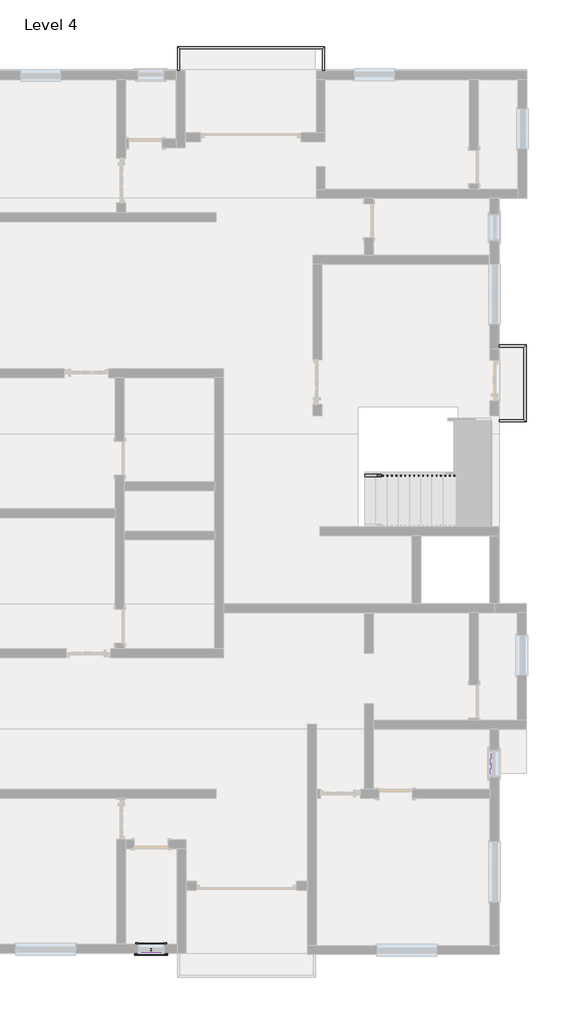
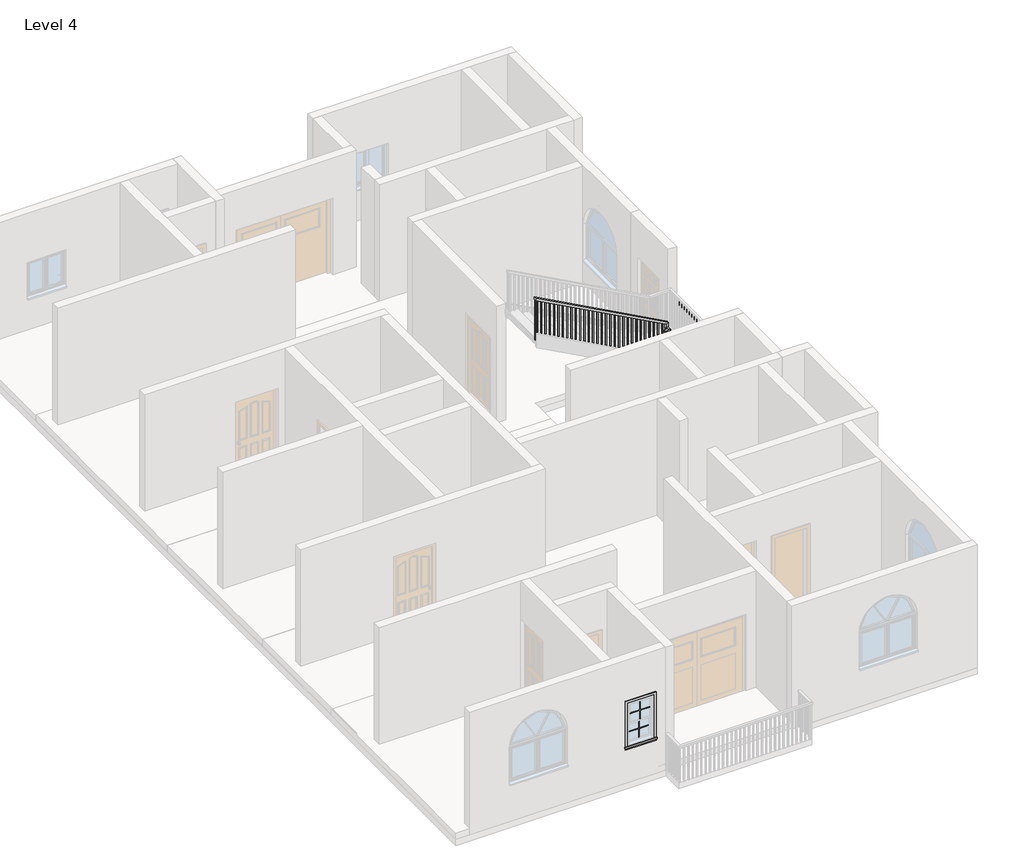
# One storey, part 6 of 7: 5 proxies, 3 railings.
"""IFC4 building model written with IfcOpenShell, lengths in millimetres."""

from ifc_helpers import new_model, si_unit, frame, origin, place, context, project, spatial, polyline, outline, extrude, faceted_brep, transform, mapped, element, save
from components import muntin_pattern_2x2_muntin_pattern_2x2_eba6c5fb, trim_window_exterior_flat_with_sill_278e6a94, trim_window_interior_flat_picture_frame_e9fd5f45

model = new_model("IFC4")

# Units and contexts
model_context = context("Model", 3, world=origin())
ifc_project = project(units=[si_unit("LENGTHUNIT", "METRE", prefix="MILLI")], contexts=[model_context])

# Site, building, storey
site = spatial("IfcSite", under=ifc_project)
building = spatial("IfcBuilding", under=site)
storey = spatial("IfcBuildingStorey", under=building, Name="Level 4", Elevation=9144.0)

# Proxies
placement = place(None, origin())
muntin_pattern_2x2_muntin_pattern_2x2_shape = muntin_pattern_2x2_muntin_pattern_2x2_eba6c5fb(model_context)
element("IfcBuildingElementProxy", 1, Name="Muntin Pattern_2x2 : Muntin Pattern_2x2", ObjectType="Muntin Pattern_2x2 : Muntin Pattern_2x2", at=placement, inside=storey, context=model_context, shape_type="MappedRepresentation", body=[
    mapped(muntin_pattern_2x2_muntin_pattern_2x2_shape, transform((5694.9140963, -6313.9537749, 10614.025), x_axis=(0.0, 1.0, 0.0), y_axis=(-1.0, 0.0, 0.0), z_axis=(0.0, 0.0, 1.0))),
])
element("IfcBuildingElementProxy", 2, Name="Muntin Pattern_2x2 : Muntin Pattern_2x2", ObjectType="Muntin Pattern_2x2 : Muntin Pattern_2x2", at=placement, inside=storey, context=model_context, shape_type="MappedRepresentation", body=[
    mapped(muntin_pattern_2x2_muntin_pattern_2x2_shape, transform((-2023.5109037, -10577.9787749, 10614.025), x_axis=(-1.0, 0.0, 0.0), y_axis=(0.0, -1.0, 0.0), z_axis=(0.0, 0.0, 1.0))),
])
element("IfcBuildingElementProxy", 3, Name="Muntin Pattern_2x2 : Muntin Pattern_2x2", ObjectType="Muntin Pattern_2x2 : Muntin Pattern_2x2", at=placement, inside=storey, context=model_context, shape_type="MappedRepresentation", body=[
    mapped(muntin_pattern_2x2_muntin_pattern_2x2_shape, transform((-2023.5109037, -10533.5287749, 10134.6), x_axis=(-1.0, 0.0, 0.0), y_axis=(0.0, -1.0, 0.0), z_axis=(0.0, 0.0, 1.0))),
])
trim_window_exterior_flat_with_sill_shape = trim_window_exterior_flat_with_sill_278e6a94(model_context)
element("IfcBuildingElementProxy", 4, Name="Trim-Window-Exterior-Flat : with Sill", ObjectType="Trim-Window-Exterior-Flat : with Sill", at=placement, inside=storey, context=model_context, shape_type="MappedRepresentation", body=[
    mapped(trim_window_exterior_flat_with_sill_shape, transform((-2023.5109037, -10612.9037749, 11125.2), x_axis=(1.0, 0.0, 0.0), y_axis=(0.0, 0.0, 1.0), z_axis=(0.0, -1.0, 0.0))),
])
trim_window_interior_flat_picture_frame_shape = trim_window_interior_flat_picture_frame_e9fd5f45(model_context)
element("IfcBuildingElementProxy", 5, Name="Trim-Window-Interior-Flat : Picture Frame", ObjectType="Trim-Window-Interior-Flat : Picture Frame", at=placement, inside=storey, context=model_context, shape_type="MappedRepresentation", body=[
    mapped(trim_window_interior_flat_picture_frame_shape, transform((-2023.5109037, -10409.7037749, 11125.2), x_axis=(-1.0, 0.0, 0.0), y_axis=(0.0, 0.0, 1.0), z_axis=(0.0, 1.0, 0.0))),
])

# Railings
element("IfcRailing", 6, ObjectType="Handrail - Rectangular", at=placement, inside=storey, context=model_context, shape_type="SolidModel", body=[
    faceted_brep([(-1426.6109037, 9402.2962251, 10058.4), (-1426.6109037, 9402.2962251, 10007.6), (-1375.8109037, 9402.2962251, 10007.6), (-1375.8109037, 9402.2962251, 10058.4), (-1426.6109037, 9948.3962251, 10058.4), (-1426.6109037, 9948.3962251, 10007.6), (-1375.8109037, 9897.5962251, 10007.6), (-1375.8109037, 9897.5962251, 10058.4), (1913.4890963, 9948.3962251, 10058.4), (1913.4890963, 9948.3962251, 10007.6), (1862.6890963, 9897.5962251, 10007.6), (1862.6890963, 9897.5962251, 10058.4), (1913.4890963, 9402.2962251, 10058.4), (1862.6890963, 9402.2962251, 10058.4), (1862.6890963, 9402.2962251, 10007.6), (1913.4890963, 9402.2962251, 10007.6)], [[[0, 1, 2, 3]], [[1, 0, 4, 5]], [[2, 1, 5, 6]], [[3, 2, 6, 7]], [[0, 3, 7, 4]], [[5, 4, 8, 9]], [[6, 5, 9, 10]], [[7, 6, 10, 11]], [[4, 7, 11, 8]], [[12, 13, 14, 15]], [[9, 8, 12, 15]], [[10, 9, 15, 14]], [[11, 10, 14, 13]], [[8, 11, 13, 12]]]),
    extrude(outline(polyline([(1878.5640963, 9424.5212251), (1897.6140963, 9424.5212251), (1897.6140963, 9405.4712251), (1878.5640963, 9405.4712251), (1878.5640963, 9424.5212251)])), frame((0.0, 0.0, 9144.0), z_axis=(0.0, 0.0, 1.0), x_axis=(1.0, 0.0, 0.0)), (0.0, 0.0, 1.0), 863.6),
    extrude(outline(polyline([(1878.5640963, 9526.1212251), (1897.6140963, 9526.1212251), (1897.6140963, 9507.0712251), (1878.5640963, 9507.0712251), (1878.5640963, 9526.1212251)])), frame((0.0, 0.0, 9144.0), z_axis=(0.0, 0.0, 1.0), x_axis=(1.0, 0.0, 0.0)), (0.0, 0.0, 1.0), 863.6),
    extrude(outline(polyline([(1878.5640963, 9627.7212251), (1897.6140963, 9627.7212251), (1897.6140963, 9608.6712251), (1878.5640963, 9608.6712251), (1878.5640963, 9627.7212251)])), frame((0.0, 0.0, 9144.0), z_axis=(0.0, 0.0, 1.0), x_axis=(1.0, 0.0, 0.0)), (0.0, 0.0, 1.0), 863.6),
    extrude(outline(polyline([(1878.5640963, 9729.3212251), (1897.6140963, 9729.3212251), (1897.6140963, 9710.2712251), (1878.5640963, 9710.2712251), (1878.5640963, 9729.3212251)])), frame((0.0, 0.0, 9144.0), z_axis=(0.0, 0.0, 1.0), x_axis=(1.0, 0.0, 0.0)), (0.0, 0.0, 1.0), 863.6),
    extrude(outline(polyline([(1878.5640963, 9830.9212251), (1897.6140963, 9830.9212251), (1897.6140963, 9811.8712251), (1878.5640963, 9811.8712251), (1878.5640963, 9830.9212251)])), frame((0.0, 0.0, 9144.0), z_axis=(0.0, 0.0, 1.0), x_axis=(1.0, 0.0, 0.0)), (0.0, 0.0, 1.0), 863.6),
    extrude(outline(polyline([(1840.4640963, 9913.4712251), (1840.4640963, 9932.5212251), (1859.5140963, 9932.5212251), (1859.5140963, 9913.4712251), (1840.4640963, 9913.4712251)])), frame((0.0, 0.0, 9144.0), z_axis=(0.0, 0.0, 1.0), x_axis=(1.0, 0.0, 0.0)), (0.0, 0.0, 1.0), 863.6),
    extrude(outline(polyline([(1738.8640963, 9913.4712251), (1738.8640963, 9932.5212251), (1757.9140963, 9932.5212251), (1757.9140963, 9913.4712251), (1738.8640963, 9913.4712251)])), frame((0.0, 0.0, 9144.0), z_axis=(0.0, 0.0, 1.0), x_axis=(1.0, 0.0, 0.0)), (0.0, 0.0, 1.0), 863.6),
    extrude(outline(polyline([(1637.2640963, 9913.4712251), (1637.2640963, 9932.5212251), (1656.3140963, 9932.5212251), (1656.3140963, 9913.4712251), (1637.2640963, 9913.4712251)])), frame((0.0, 0.0, 9144.0), z_axis=(0.0, 0.0, 1.0), x_axis=(1.0, 0.0, 0.0)), (0.0, 0.0, 1.0), 863.6),
    extrude(outline(polyline([(1535.6640963, 9913.4712251), (1535.6640963, 9932.5212251), (1554.7140963, 9932.5212251), (1554.7140963, 9913.4712251), (1535.6640963, 9913.4712251)])), frame((0.0, 0.0, 9144.0), z_axis=(0.0, 0.0, 1.0), x_axis=(1.0, 0.0, 0.0)), (0.0, 0.0, 1.0), 863.6),
    extrude(outline(polyline([(1434.0640963, 9913.4712251), (1434.0640963, 9932.5212251), (1453.1140963, 9932.5212251), (1453.1140963, 9913.4712251), (1434.0640963, 9913.4712251)])), frame((0.0, 0.0, 9144.0), z_axis=(0.0, 0.0, 1.0), x_axis=(1.0, 0.0, 0.0)), (0.0, 0.0, 1.0), 863.6),
    extrude(outline(polyline([(1332.4640963, 9913.4712251), (1332.4640963, 9932.5212251), (1351.5140963, 9932.5212251), (1351.5140963, 9913.4712251), (1332.4640963, 9913.4712251)])), frame((0.0, 0.0, 9144.0), z_axis=(0.0, 0.0, 1.0), x_axis=(1.0, 0.0, 0.0)), (0.0, 0.0, 1.0), 863.6),
    extrude(outline(polyline([(1230.8640963, 9913.4712251), (1230.8640963, 9932.5212251), (1249.9140963, 9932.5212251), (1249.9140963, 9913.4712251), (1230.8640963, 9913.4712251)])), frame((0.0, 0.0, 9144.0), z_axis=(0.0, 0.0, 1.0), x_axis=(1.0, 0.0, 0.0)), (0.0, 0.0, 1.0), 863.6),
    extrude(outline(polyline([(1129.2640963, 9913.4712251), (1129.2640963, 9932.5212251), (1148.3140963, 9932.5212251), (1148.3140963, 9913.4712251), (1129.2640963, 9913.4712251)])), frame((0.0, 0.0, 9144.0), z_axis=(0.0, 0.0, 1.0), x_axis=(1.0, 0.0, 0.0)), (0.0, 0.0, 1.0), 863.6),
    extrude(outline(polyline([(1027.6640963, 9913.4712251), (1027.6640963, 9932.5212251), (1046.7140963, 9932.5212251), (1046.7140963, 9913.4712251), (1027.6640963, 9913.4712251)])), frame((0.0, 0.0, 9144.0), z_axis=(0.0, 0.0, 1.0), x_axis=(1.0, 0.0, 0.0)), (0.0, 0.0, 1.0), 863.6),
    extrude(outline(polyline([(926.0640963, 9913.4712251), (926.0640963, 9932.5212251), (945.1140963, 9932.5212251), (945.1140963, 9913.4712251), (926.0640963, 9913.4712251)])), frame((0.0, 0.0, 9144.0), z_axis=(0.0, 0.0, 1.0), x_axis=(1.0, 0.0, 0.0)), (0.0, 0.0, 1.0), 863.6),
    extrude(outline(polyline([(824.4640963, 9913.4712251), (824.4640963, 9932.5212251), (843.5140963, 9932.5212251), (843.5140963, 9913.4712251), (824.4640963, 9913.4712251)])), frame((0.0, 0.0, 9144.0), z_axis=(0.0, 0.0, 1.0), x_axis=(1.0, 0.0, 0.0)), (0.0, 0.0, 1.0), 863.6),
    extrude(outline(polyline([(722.8640963, 9913.4712251), (722.8640963, 9932.5212251), (741.9140963, 9932.5212251), (741.9140963, 9913.4712251), (722.8640963, 9913.4712251)])), frame((0.0, 0.0, 9144.0), z_axis=(0.0, 0.0, 1.0), x_axis=(1.0, 0.0, 0.0)), (0.0, 0.0, 1.0), 863.6),
    extrude(outline(polyline([(621.2640963, 9913.4712251), (621.2640963, 9932.5212251), (640.3140963, 9932.5212251), (640.3140963, 9913.4712251), (621.2640963, 9913.4712251)])), frame((0.0, 0.0, 9144.0), z_axis=(0.0, 0.0, 1.0), x_axis=(1.0, 0.0, 0.0)), (0.0, 0.0, 1.0), 863.6),
    extrude(outline(polyline([(519.6640963, 9913.4712251), (519.6640963, 9932.5212251), (538.7140963, 9932.5212251), (538.7140963, 9913.4712251), (519.6640963, 9913.4712251)])), frame((0.0, 0.0, 9144.0), z_axis=(0.0, 0.0, 1.0), x_axis=(1.0, 0.0, 0.0)), (0.0, 0.0, 1.0), 863.6),
    extrude(outline(polyline([(418.0640963, 9913.4712251), (418.0640963, 9932.5212251), (437.1140963, 9932.5212251), (437.1140963, 9913.4712251), (418.0640963, 9913.4712251)])), frame((0.0, 0.0, 9144.0), z_axis=(0.0, 0.0, 1.0), x_axis=(1.0, 0.0, 0.0)), (0.0, 0.0, 1.0), 863.6),
    extrude(outline(polyline([(316.4640963, 9913.4712251), (316.4640963, 9932.5212251), (335.5140963, 9932.5212251), (335.5140963, 9913.4712251), (316.4640963, 9913.4712251)])), frame((0.0, 0.0, 9144.0), z_axis=(0.0, 0.0, 1.0), x_axis=(1.0, 0.0, 0.0)), (0.0, 0.0, 1.0), 863.6),
    extrude(outline(polyline([(214.8640963, 9913.4712251), (214.8640963, 9932.5212251), (233.9140963, 9932.5212251), (233.9140963, 9913.4712251), (214.8640963, 9913.4712251)])), frame((0.0, 0.0, 9144.0), z_axis=(0.0, 0.0, 1.0), x_axis=(1.0, 0.0, 0.0)), (0.0, 0.0, 1.0), 863.6),
    extrude(outline(polyline([(113.2640963, 9913.4712251), (113.2640963, 9932.5212251), (132.3140963, 9932.5212251), (132.3140963, 9913.4712251), (113.2640963, 9913.4712251)])), frame((0.0, 0.0, 9144.0), z_axis=(0.0, 0.0, 1.0), x_axis=(1.0, 0.0, 0.0)), (0.0, 0.0, 1.0), 863.6),
    extrude(outline(polyline([(11.6640963, 9913.4712251), (11.6640963, 9932.5212251), (30.7140963, 9932.5212251), (30.7140963, 9913.4712251), (11.6640963, 9913.4712251)])), frame((0.0, 0.0, 9144.0), z_axis=(0.0, 0.0, 1.0), x_axis=(1.0, 0.0, 0.0)), (0.0, 0.0, 1.0), 863.6),
    extrude(outline(polyline([(-89.9359037, 9913.4712251), (-89.9359037, 9932.5212251), (-70.8859037, 9932.5212251), (-70.8859037, 9913.4712251), (-89.9359037, 9913.4712251)])), frame((0.0, 0.0, 9144.0), z_axis=(0.0, 0.0, 1.0), x_axis=(1.0, 0.0, 0.0)), (0.0, 0.0, 1.0), 863.6),
    extrude(outline(polyline([(-191.5359037, 9913.4712251), (-191.5359037, 9932.5212251), (-172.4859037, 9932.5212251), (-172.4859037, 9913.4712251), (-191.5359037, 9913.4712251)])), frame((0.0, 0.0, 9144.0), z_axis=(0.0, 0.0, 1.0), x_axis=(1.0, 0.0, 0.0)), (0.0, 0.0, 1.0), 863.6),
    extrude(outline(polyline([(-293.1359037, 9913.4712251), (-293.1359037, 9932.5212251), (-274.0859037, 9932.5212251), (-274.0859037, 9913.4712251), (-293.1359037, 9913.4712251)])), frame((0.0, 0.0, 9144.0), z_axis=(0.0, 0.0, 1.0), x_axis=(1.0, 0.0, 0.0)), (0.0, 0.0, 1.0), 863.6),
    extrude(outline(polyline([(-394.7359037, 9913.4712251), (-394.7359037, 9932.5212251), (-375.6859037, 9932.5212251), (-375.6859037, 9913.4712251), (-394.7359037, 9913.4712251)])), frame((0.0, 0.0, 9144.0), z_axis=(0.0, 0.0, 1.0), x_axis=(1.0, 0.0, 0.0)), (0.0, 0.0, 1.0), 863.6),
    extrude(outline(polyline([(-496.3359037, 9913.4712251), (-496.3359037, 9932.5212251), (-477.2859037, 9932.5212251), (-477.2859037, 9913.4712251), (-496.3359037, 9913.4712251)])), frame((0.0, 0.0, 9144.0), z_axis=(0.0, 0.0, 1.0), x_axis=(1.0, 0.0, 0.0)), (0.0, 0.0, 1.0), 863.6),
    extrude(outline(polyline([(-597.9359037, 9913.4712251), (-597.9359037, 9932.5212251), (-578.8859037, 9932.5212251), (-578.8859037, 9913.4712251), (-597.9359037, 9913.4712251)])), frame((0.0, 0.0, 9144.0), z_axis=(0.0, 0.0, 1.0), x_axis=(1.0, 0.0, 0.0)), (0.0, 0.0, 1.0), 863.6),
    extrude(outline(polyline([(-699.5359037, 9913.4712251), (-699.5359037, 9932.5212251), (-680.4859037, 9932.5212251), (-680.4859037, 9913.4712251), (-699.5359037, 9913.4712251)])), frame((0.0, 0.0, 9144.0), z_axis=(0.0, 0.0, 1.0), x_axis=(1.0, 0.0, 0.0)), (0.0, 0.0, 1.0), 863.6),
    extrude(outline(polyline([(-801.1359037, 9913.4712251), (-801.1359037, 9932.5212251), (-782.0859037, 9932.5212251), (-782.0859037, 9913.4712251), (-801.1359037, 9913.4712251)])), frame((0.0, 0.0, 9144.0), z_axis=(0.0, 0.0, 1.0), x_axis=(1.0, 0.0, 0.0)), (0.0, 0.0, 1.0), 863.6),
    extrude(outline(polyline([(-902.7359037, 9913.4712251), (-902.7359037, 9932.5212251), (-883.6859037, 9932.5212251), (-883.6859037, 9913.4712251), (-902.7359037, 9913.4712251)])), frame((0.0, 0.0, 9144.0), z_axis=(0.0, 0.0, 1.0), x_axis=(1.0, 0.0, 0.0)), (0.0, 0.0, 1.0), 863.6),
    extrude(outline(polyline([(-1004.3359037, 9913.4712251), (-1004.3359037, 9932.5212251), (-985.2859037, 9932.5212251), (-985.2859037, 9913.4712251), (-1004.3359037, 9913.4712251)])), frame((0.0, 0.0, 9144.0), z_axis=(0.0, 0.0, 1.0), x_axis=(1.0, 0.0, 0.0)), (0.0, 0.0, 1.0), 863.6),
    extrude(outline(polyline([(-1105.9359037, 9913.4712251), (-1105.9359037, 9932.5212251), (-1086.8859037, 9932.5212251), (-1086.8859037, 9913.4712251), (-1105.9359037, 9913.4712251)])), frame((0.0, 0.0, 9144.0), z_axis=(0.0, 0.0, 1.0), x_axis=(1.0, 0.0, 0.0)), (0.0, 0.0, 1.0), 863.6),
    extrude(outline(polyline([(-1207.5359037, 9913.4712251), (-1207.5359037, 9932.5212251), (-1188.4859037, 9932.5212251), (-1188.4859037, 9913.4712251), (-1207.5359037, 9913.4712251)])), frame((0.0, 0.0, 9144.0), z_axis=(0.0, 0.0, 1.0), x_axis=(1.0, 0.0, 0.0)), (0.0, 0.0, 1.0), 863.6),
    extrude(outline(polyline([(-1309.1359037, 9913.4712251), (-1309.1359037, 9932.5212251), (-1290.0859037, 9932.5212251), (-1290.0859037, 9913.4712251), (-1309.1359037, 9913.4712251)])), frame((0.0, 0.0, 9144.0), z_axis=(0.0, 0.0, 1.0), x_axis=(1.0, 0.0, 0.0)), (0.0, 0.0, 1.0), 863.6),
    extrude(outline(polyline([(-1391.6859037, 9900.7712251), (-1410.7359037, 9900.7712251), (-1410.7359037, 9919.8212251), (-1391.6859037, 9919.8212251), (-1391.6859037, 9900.7712251)])), frame((0.0, 0.0, 9144.0), z_axis=(0.0, 0.0, 1.0), x_axis=(1.0, 0.0, 0.0)), (0.0, 0.0, 1.0), 863.6),
    extrude(outline(polyline([(-1391.6859037, 9799.1712251), (-1410.7359037, 9799.1712251), (-1410.7359037, 9818.2212251), (-1391.6859037, 9818.2212251), (-1391.6859037, 9799.1712251)])), frame((0.0, 0.0, 9144.0), z_axis=(0.0, 0.0, 1.0), x_axis=(1.0, 0.0, 0.0)), (0.0, 0.0, 1.0), 863.6),
    extrude(outline(polyline([(-1391.6859037, 9697.5712251), (-1410.7359037, 9697.5712251), (-1410.7359037, 9716.6212251), (-1391.6859037, 9716.6212251), (-1391.6859037, 9697.5712251)])), frame((0.0, 0.0, 9144.0), z_axis=(0.0, 0.0, 1.0), x_axis=(1.0, 0.0, 0.0)), (0.0, 0.0, 1.0), 863.6),
    extrude(outline(polyline([(-1391.6859037, 9595.9712251), (-1410.7359037, 9595.9712251), (-1410.7359037, 9615.0212251), (-1391.6859037, 9615.0212251), (-1391.6859037, 9595.9712251)])), frame((0.0, 0.0, 9144.0), z_axis=(0.0, 0.0, 1.0), x_axis=(1.0, 0.0, 0.0)), (0.0, 0.0, 1.0), 863.6),
    extrude(outline(polyline([(-1391.6859037, 9494.3712251), (-1410.7359037, 9494.3712251), (-1410.7359037, 9513.4212251), (-1391.6859037, 9513.4212251), (-1391.6859037, 9494.3712251)])), frame((0.0, 0.0, 9144.0), z_axis=(0.0, 0.0, 1.0), x_axis=(1.0, 0.0, 0.0)), (0.0, 0.0, 1.0), 863.6),
    extrude(outline(polyline([(1878.5640963, 9913.4712251), (1878.5640963, 9932.5212251), (1897.6140963, 9932.5212251), (1897.6140963, 9913.4712251), (1878.5640963, 9913.4712251)])), frame((0.0, 0.0, 9144.0), z_axis=(0.0, 0.0, 1.0), x_axis=(1.0, 0.0, 0.0)), (0.0, 0.0, 1.0), 863.6),
    extrude(outline(polyline([(-1391.6859037, 9913.4712251), (-1410.7359037, 9913.4712251), (-1410.7359037, 9932.5212251), (-1391.6859037, 9932.5212251), (-1391.6859037, 9913.4712251)])), frame((0.0, 0.0, 9144.0), z_axis=(0.0, 0.0, 1.0), x_axis=(1.0, 0.0, 0.0)), (0.0, 0.0, 1.0), 863.6),
    extrude(outline(polyline([(1878.5640963, 9421.3462251), (1897.6140963, 9421.3462251), (1897.6140963, 9402.2962251), (1878.5640963, 9402.2962251), (1878.5640963, 9421.3462251)])), frame((0.0, 0.0, 9144.0), z_axis=(0.0, 0.0, 1.0), x_axis=(1.0, 0.0, 0.0)), (0.0, 0.0, 1.0), 863.6),
    extrude(outline(polyline([(-1391.6859037, 9402.2962251), (-1410.7359037, 9402.2962251), (-1410.7359037, 9421.3462251), (-1391.6859037, 9421.3462251), (-1391.6859037, 9402.2962251)])), frame((0.0, 0.0, 9144.0), z_axis=(0.0, 0.0, 1.0), x_axis=(1.0, 0.0, 0.0)), (0.0, 0.0, 1.0), 863.6),
])
element("IfcRailing", 7, ObjectType="Handrail - Rectangular", at=placement, inside=storey, context=model_context, shape_type="SolidModel", body=[
    faceted_brep([(5863.1890963, 3183.81308, 10058.4), (5863.1890963, 3183.81308, 10007.6), (5863.1890963, 3133.01308, 10007.6), (5863.1890963, 3133.01308, 10058.4), (6485.4890963, 3183.81308, 10058.4), (6485.4890963, 3183.81308, 10007.6), (6434.6890963, 3133.01308, 10007.6), (6434.6890963, 3133.01308, 10058.4), (6485.4890963, 1439.3962251, 10058.4), (6485.4890963, 1439.3962251, 10007.6), (6434.6890963, 1490.1962251, 10007.6), (6434.6890963, 1490.1962251, 10058.4), (5875.8890963, 1439.3962251, 10058.4), (5875.8890963, 1490.1962251, 10058.4), (5875.8890963, 1490.1962251, 10007.6), (5875.8890963, 1439.3962251, 10007.6)], [[[0, 1, 2, 3]], [[1, 0, 4, 5]], [[2, 1, 5, 6]], [[3, 2, 6, 7]], [[0, 3, 7, 4]], [[5, 4, 8, 9]], [[6, 5, 9, 10]], [[7, 6, 10, 11]], [[4, 7, 11, 8]], [[12, 13, 14, 15]], [[9, 8, 12, 15]], [[10, 9, 15, 14]], [[11, 10, 14, 13]], [[8, 11, 13, 12]]]),
    extrude(outline(polyline([(5961.6140963, 1474.3212251), (5961.6140963, 1455.2712251), (5942.5640963, 1455.2712251), (5942.5640963, 1474.3212251), (5961.6140963, 1474.3212251)])), frame((0.0, 0.0, 9144.0), z_axis=(0.0, 0.0, 1.0), x_axis=(1.0, 0.0, 0.0)), (0.0, 0.0, 1.0), 863.6),
    extrude(outline(polyline([(6063.2140963, 1474.3212251), (6063.2140963, 1455.2712251), (6044.1640963, 1455.2712251), (6044.1640963, 1474.3212251), (6063.2140963, 1474.3212251)])), frame((0.0, 0.0, 9144.0), z_axis=(0.0, 0.0, 1.0), x_axis=(1.0, 0.0, 0.0)), (0.0, 0.0, 1.0), 863.6),
    extrude(outline(polyline([(6164.8140963, 1474.3212251), (6164.8140963, 1455.2712251), (6145.7640963, 1455.2712251), (6145.7640963, 1474.3212251), (6164.8140963, 1474.3212251)])), frame((0.0, 0.0, 9144.0), z_axis=(0.0, 0.0, 1.0), x_axis=(1.0, 0.0, 0.0)), (0.0, 0.0, 1.0), 863.6),
    extrude(outline(polyline([(6266.4140963, 1474.3212251), (6266.4140963, 1455.2712251), (6247.3640963, 1455.2712251), (6247.3640963, 1474.3212251), (6266.4140963, 1474.3212251)])), frame((0.0, 0.0, 9144.0), z_axis=(0.0, 0.0, 1.0), x_axis=(1.0, 0.0, 0.0)), (0.0, 0.0, 1.0), 863.6),
    extrude(outline(polyline([(6368.0140963, 1474.3212251), (6368.0140963, 1455.2712251), (6348.9640963, 1455.2712251), (6348.9640963, 1474.3212251), (6368.0140963, 1474.3212251)])), frame((0.0, 0.0, 9144.0), z_axis=(0.0, 0.0, 1.0), x_axis=(1.0, 0.0, 0.0)), (0.0, 0.0, 1.0), 863.6),
    extrude(outline(polyline([(6450.5640963, 1542.33808), (6469.6140963, 1542.33808), (6469.6140963, 1523.28808), (6450.5640963, 1523.28808), (6450.5640963, 1542.33808)])), frame((0.0, 0.0, 9144.0), z_axis=(0.0, 0.0, 1.0), x_axis=(1.0, 0.0, 0.0)), (0.0, 0.0, 1.0), 863.6),
    extrude(outline(polyline([(6450.5640963, 1643.93808), (6469.6140963, 1643.93808), (6469.6140963, 1624.88808), (6450.5640963, 1624.88808), (6450.5640963, 1643.93808)])), frame((0.0, 0.0, 9144.0), z_axis=(0.0, 0.0, 1.0), x_axis=(1.0, 0.0, 0.0)), (0.0, 0.0, 1.0), 863.6),
    extrude(outline(polyline([(6450.5640963, 1745.53808), (6469.6140963, 1745.53808), (6469.6140963, 1726.48808), (6450.5640963, 1726.48808), (6450.5640963, 1745.53808)])), frame((0.0, 0.0, 9144.0), z_axis=(0.0, 0.0, 1.0), x_axis=(1.0, 0.0, 0.0)), (0.0, 0.0, 1.0), 863.6),
    extrude(outline(polyline([(6450.5640963, 1847.13808), (6469.6140963, 1847.13808), (6469.6140963, 1828.08808), (6450.5640963, 1828.08808), (6450.5640963, 1847.13808)])), frame((0.0, 0.0, 9144.0), z_axis=(0.0, 0.0, 1.0), x_axis=(1.0, 0.0, 0.0)), (0.0, 0.0, 1.0), 863.6),
    extrude(outline(polyline([(6450.5640963, 1948.73808), (6469.6140963, 1948.73808), (6469.6140963, 1929.68808), (6450.5640963, 1929.68808), (6450.5640963, 1948.73808)])), frame((0.0, 0.0, 9144.0), z_axis=(0.0, 0.0, 1.0), x_axis=(1.0, 0.0, 0.0)), (0.0, 0.0, 1.0), 863.6),
    extrude(outline(polyline([(6450.5640963, 2050.33808), (6469.6140963, 2050.33808), (6469.6140963, 2031.28808), (6450.5640963, 2031.28808), (6450.5640963, 2050.33808)])), frame((0.0, 0.0, 9144.0), z_axis=(0.0, 0.0, 1.0), x_axis=(1.0, 0.0, 0.0)), (0.0, 0.0, 1.0), 863.6),
    extrude(outline(polyline([(6450.5640963, 2151.93808), (6469.6140963, 2151.93808), (6469.6140963, 2132.88808), (6450.5640963, 2132.88808), (6450.5640963, 2151.93808)])), frame((0.0, 0.0, 9144.0), z_axis=(0.0, 0.0, 1.0), x_axis=(1.0, 0.0, 0.0)), (0.0, 0.0, 1.0), 863.6),
    extrude(outline(polyline([(6450.5640963, 2253.53808), (6469.6140963, 2253.53808), (6469.6140963, 2234.48808), (6450.5640963, 2234.48808), (6450.5640963, 2253.53808)])), frame((0.0, 0.0, 9144.0), z_axis=(0.0, 0.0, 1.0), x_axis=(1.0, 0.0, 0.0)), (0.0, 0.0, 1.0), 863.6),
    extrude(outline(polyline([(6450.5640963, 2355.13808), (6469.6140963, 2355.13808), (6469.6140963, 2336.08808), (6450.5640963, 2336.08808), (6450.5640963, 2355.13808)])), frame((0.0, 0.0, 9144.0), z_axis=(0.0, 0.0, 1.0), x_axis=(1.0, 0.0, 0.0)), (0.0, 0.0, 1.0), 863.6),
    extrude(outline(polyline([(6450.5640963, 2456.73808), (6469.6140963, 2456.73808), (6469.6140963, 2437.68808), (6450.5640963, 2437.68808), (6450.5640963, 2456.73808)])), frame((0.0, 0.0, 9144.0), z_axis=(0.0, 0.0, 1.0), x_axis=(1.0, 0.0, 0.0)), (0.0, 0.0, 1.0), 863.6),
    extrude(outline(polyline([(6450.5640963, 2558.33808), (6469.6140963, 2558.33808), (6469.6140963, 2539.28808), (6450.5640963, 2539.28808), (6450.5640963, 2558.33808)])), frame((0.0, 0.0, 9144.0), z_axis=(0.0, 0.0, 1.0), x_axis=(1.0, 0.0, 0.0)), (0.0, 0.0, 1.0), 863.6),
    extrude(outline(polyline([(6450.5640963, 2659.93808), (6469.6140963, 2659.93808), (6469.6140963, 2640.88808), (6450.5640963, 2640.88808), (6450.5640963, 2659.93808)])), frame((0.0, 0.0, 9144.0), z_axis=(0.0, 0.0, 1.0), x_axis=(1.0, 0.0, 0.0)), (0.0, 0.0, 1.0), 863.6),
    extrude(outline(polyline([(6450.5640963, 2761.53808), (6469.6140963, 2761.53808), (6469.6140963, 2742.48808), (6450.5640963, 2742.48808), (6450.5640963, 2761.53808)])), frame((0.0, 0.0, 9144.0), z_axis=(0.0, 0.0, 1.0), x_axis=(1.0, 0.0, 0.0)), (0.0, 0.0, 1.0), 863.6),
    extrude(outline(polyline([(6450.5640963, 2863.13808), (6469.6140963, 2863.13808), (6469.6140963, 2844.08808), (6450.5640963, 2844.08808), (6450.5640963, 2863.13808)])), frame((0.0, 0.0, 9144.0), z_axis=(0.0, 0.0, 1.0), x_axis=(1.0, 0.0, 0.0)), (0.0, 0.0, 1.0), 863.6),
    extrude(outline(polyline([(6450.5640963, 2964.73808), (6469.6140963, 2964.73808), (6469.6140963, 2945.68808), (6450.5640963, 2945.68808), (6450.5640963, 2964.73808)])), frame((0.0, 0.0, 9144.0), z_axis=(0.0, 0.0, 1.0), x_axis=(1.0, 0.0, 0.0)), (0.0, 0.0, 1.0), 863.6),
    extrude(outline(polyline([(6450.5640963, 3066.33808), (6469.6140963, 3066.33808), (6469.6140963, 3047.28808), (6450.5640963, 3047.28808), (6450.5640963, 3066.33808)])), frame((0.0, 0.0, 9144.0), z_axis=(0.0, 0.0, 1.0), x_axis=(1.0, 0.0, 0.0)), (0.0, 0.0, 1.0), 863.6),
    extrude(outline(polyline([(6361.6640963, 3148.88808), (6361.6640963, 3167.93808), (6380.7140963, 3167.93808), (6380.7140963, 3148.88808), (6361.6640963, 3148.88808)])), frame((0.0, 0.0, 9144.0), z_axis=(0.0, 0.0, 1.0), x_axis=(1.0, 0.0, 0.0)), (0.0, 0.0, 1.0), 863.6),
    extrude(outline(polyline([(6260.0640963, 3148.88808), (6260.0640963, 3167.93808), (6279.1140963, 3167.93808), (6279.1140963, 3148.88808), (6260.0640963, 3148.88808)])), frame((0.0, 0.0, 9144.0), z_axis=(0.0, 0.0, 1.0), x_axis=(1.0, 0.0, 0.0)), (0.0, 0.0, 1.0), 863.6),
    extrude(outline(polyline([(6158.4640963, 3148.88808), (6158.4640963, 3167.93808), (6177.5140963, 3167.93808), (6177.5140963, 3148.88808), (6158.4640963, 3148.88808)])), frame((0.0, 0.0, 9144.0), z_axis=(0.0, 0.0, 1.0), x_axis=(1.0, 0.0, 0.0)), (0.0, 0.0, 1.0), 863.6),
    extrude(outline(polyline([(6056.8640963, 3148.88808), (6056.8640963, 3167.93808), (6075.9140963, 3167.93808), (6075.9140963, 3148.88808), (6056.8640963, 3148.88808)])), frame((0.0, 0.0, 9144.0), z_axis=(0.0, 0.0, 1.0), x_axis=(1.0, 0.0, 0.0)), (0.0, 0.0, 1.0), 863.6),
    extrude(outline(polyline([(5955.2640963, 3148.88808), (5955.2640963, 3167.93808), (5974.3140963, 3167.93808), (5974.3140963, 3148.88808), (5955.2640963, 3148.88808)])), frame((0.0, 0.0, 9144.0), z_axis=(0.0, 0.0, 1.0), x_axis=(1.0, 0.0, 0.0)), (0.0, 0.0, 1.0), 863.6),
    extrude(outline(polyline([(6450.5640963, 1474.3212251), (6469.6140963, 1474.3212251), (6469.6140963, 1455.2712251), (6450.5640963, 1455.2712251), (6450.5640963, 1474.3212251)])), frame((0.0, 0.0, 9144.0), z_axis=(0.0, 0.0, 1.0), x_axis=(1.0, 0.0, 0.0)), (0.0, 0.0, 1.0), 863.6),
    extrude(outline(polyline([(6450.5640963, 3148.88808), (6450.5640963, 3167.93808), (6469.6140963, 3167.93808), (6469.6140963, 3148.88808), (6450.5640963, 3148.88808)])), frame((0.0, 0.0, 9144.0), z_axis=(0.0, 0.0, 1.0), x_axis=(1.0, 0.0, 0.0)), (0.0, 0.0, 1.0), 863.6),
    extrude(outline(polyline([(5894.9390963, 1474.3212251), (5894.9390963, 1455.2712251), (5875.8890963, 1455.2712251), (5875.8890963, 1474.3212251), (5894.9390963, 1474.3212251)])), frame((0.0, 0.0, 9144.0), z_axis=(0.0, 0.0, 1.0), x_axis=(1.0, 0.0, 0.0)), (0.0, 0.0, 1.0), 863.6),
    extrude(outline(polyline([(5863.1890963, 3148.88808), (5863.1890963, 3167.93808), (5882.2390963, 3167.93808), (5882.2390963, 3148.88808), (5863.1890963, 3148.88808)])), frame((0.0, 0.0, 9144.0), z_axis=(0.0, 0.0, 1.0), x_axis=(1.0, 0.0, 0.0)), (0.0, 0.0, 1.0), 863.6),
])
element("IfcRailing", 8, ObjectType="Handrail - Rectangular", at=placement, inside=storey, context=model_context, shape_type="SolidModel", body=[
    faceted_brep([(2827.8890963, 245.5962251, 10196.9454545), (2827.8890963, 245.5962251, 10139.2159002), (2827.8890963, 194.7962251, 10139.2159002), (2827.8890963, 194.7962251, 10196.9454545), (4804.8326586, 245.5962251, 11264.1734827), (4855.6326586, 245.5962251, 11233.8676671), (4855.6326586, 194.7962251, 11233.8676671), (4804.8326586, 194.7962251, 11264.1734827), (4804.8326586, 245.5962251, 11305.3090909), (4855.6326586, 245.5962251, 11254.5090909), (4855.6326586, 194.7962251, 11254.5090909), (4804.8326586, 194.7962251, 11305.3090909), (4881.0326586, 245.5962251, 11305.3090909), (4881.0326586, 245.5962251, 11254.5090909), (4931.8326586, 194.7962251, 11254.5090909), (4931.8326586, 194.7962251, 11305.3090909), (4881.0326586, 296.3962251, 11305.3090909), (4931.8326586, 296.3962251, 11305.3090909), (4931.8326586, 347.1962251, 11254.5090909), (4881.0326586, 347.1962251, 11254.5090909)], [[[0, 1, 2, 3]], [[1, 0, 4, 5]], [[2, 1, 5, 6]], [[3, 2, 6, 7]], [[0, 3, 7, 4]], [[5, 4, 8, 9]], [[6, 5, 9, 10]], [[7, 6, 10, 11]], [[4, 7, 11, 8]], [[9, 8, 12, 13]], [[10, 9, 13, 14]], [[11, 10, 14, 15]], [[8, 11, 15, 12]], [[16, 17, 18, 19]], [[13, 12, 16, 19]], [[14, 13, 19, 18]], [[15, 14, 18, 17]], [[12, 15, 17, 16]]]),
    faceted_brep([(4931.8326586, 296.3962251, 11416.3363446), (4881.0326586, 296.3962251, 11386.0800582), (4881.0326586, 347.1962251, 11386.0800582), (4931.8326586, 347.1962251, 11416.3363446), (1811.8890963, 296.3962251, 13106.4), (1811.8890963, 347.1962251, 13106.4), (1811.8890963, 347.1962251, 13048.6255127), (1811.8890963, 296.3962251, 13048.6255127)], [[[0, 1, 2, 3]], [[4, 5, 6, 7]], [[1, 0, 4, 7]], [[2, 1, 7, 6]], [[3, 2, 6, 5]], [[0, 3, 5, 4]]]),
    faceted_brep([(4881.0326586, 296.3962251, 11305.3090909), (4881.0326586, 347.1962251, 11254.5090909), (4931.8326586, 347.1962251, 11254.5090909), (4931.8326586, 296.3962251, 11305.3090909), (4881.0326586, 296.3962251, 11386.0800582), (4931.8326586, 296.3962251, 11416.3363446), (4931.8326586, 347.1962251, 11416.3363446), (4881.0326586, 347.1962251, 11386.0800582)], [[[0, 1, 2, 3]], [[4, 5, 6, 7]], [[1, 0, 4, 7]], [[2, 1, 7, 6]], [[3, 2, 6, 5]], [[0, 3, 5, 4]]]),
    extrude(outline(polyline([(13028.5726735, 1848.9076586), (12053.4545455, 1848.9076586), (12053.4545455, 1867.9576586), (13018.2533481, 1867.9576586), (13028.5726735, 1848.9076586)])), frame((0.0, 312.2712251, 0.0), z_axis=(0.0, 1.0, 0.0), x_axis=(0.0, 0.0, 1.0)), (0.0, 0.0, 1.0), 19.05),
    extrude(outline(polyline([(12973.5362717, 1950.5076586), (12053.4545455, 1950.5076586), (12053.4545455, 1969.5576586), (12963.2169464, 1969.5576586), (12973.5362717, 1950.5076586)])), frame((0.0, 312.2712251, 0.0), z_axis=(0.0, 1.0, 0.0), x_axis=(0.0, 0.0, 1.0)), (0.0, 0.0, 1.0), 19.05),
    extrude(outline(polyline([(12918.4998699, 2052.1076586), (12053.4545455, 2052.1076586), (12053.4545455, 2071.1576586), (12908.1805446, 2071.1576586), (12918.4998699, 2052.1076586)])), frame((0.0, 312.2712251, 0.0), z_axis=(0.0, 1.0, 0.0), x_axis=(0.0, 0.0, 1.0)), (0.0, 0.0, 1.0), 19.05),
    extrude(outline(polyline([(12863.5508544, 2153.7076586), (11914.9090909, 2153.7076586), (11914.9090909, 2172.7576586), (12853.2669524, 2172.7576586), (12863.5508544, 2153.7076586)])), frame((0.0, 312.2712251, 0.0), z_axis=(0.0, 1.0, 0.0), x_axis=(0.0, 0.0, 1.0)), (0.0, 0.0, 1.0), 19.05),
    extrude(outline(polyline([(12808.4270664, 2255.3076586), (11914.9090909, 2255.3076586), (11914.9090909, 2274.3576586), (12798.1077411, 2274.3576586), (12808.4270664, 2255.3076586)])), frame((0.0, 312.2712251, 0.0), z_axis=(0.0, 1.0, 0.0), x_axis=(0.0, 0.0, 1.0)), (0.0, 0.0, 1.0), 19.05),
    extrude(outline(polyline([(12753.3906646, 2356.9076586), (11776.3636364, 2356.9076586), (11776.3636364, 2375.9576586), (12743.0713393, 2375.9576586), (12753.3906646, 2356.9076586)])), frame((0.0, 312.2712251, 0.0), z_axis=(0.0, 1.0, 0.0), x_axis=(0.0, 0.0, 1.0)), (0.0, 0.0, 1.0), 19.05),
    extrude(outline(polyline([(12698.3542629, 2458.5076586), (11776.3636364, 2458.5076586), (11776.3636364, 2477.5576586), (12688.0349375, 2477.5576586), (12698.3542629, 2458.5076586)])), frame((0.0, 312.2712251, 0.0), z_axis=(0.0, 1.0, 0.0), x_axis=(0.0, 0.0, 1.0)), (0.0, 0.0, 1.0), 19.05),
    extrude(outline(polyline([(12643.3084744, 2560.1076586), (11776.3636364, 2560.1076586), (11776.3636364, 2579.1576586), (12632.9891491, 2579.1576586), (12643.3084744, 2560.1076586)])), frame((0.0, 312.2712251, 0.0), z_axis=(0.0, 1.0, 0.0), x_axis=(0.0, 0.0, 1.0)), (0.0, 0.0, 1.0), 19.05),
    extrude(outline(polyline([(12588.2814593, 2661.7076586), (11637.8181818, 2661.7076586), (11637.8181818, 2680.7576586), (12577.962134, 2680.7576586), (12588.2814593, 2661.7076586)])), frame((0.0, 312.2712251, 0.0), z_axis=(0.0, 1.0, 0.0), x_axis=(0.0, 0.0, 1.0)), (0.0, 0.0, 1.0), 19.05),
    extrude(outline(polyline([(12533.2450575, 2763.3076586), (11637.8181818, 2763.3076586), (11637.8181818, 2782.3576586), (12522.9257322, 2782.3576586), (12533.2450575, 2763.3076586)])), frame((0.0, 312.2712251, 0.0), z_axis=(0.0, 1.0, 0.0), x_axis=(0.0, 0.0, 1.0)), (0.0, 0.0, 1.0), 19.05),
    extrude(outline(polyline([(12478.2086558, 2864.9076586), (11499.2727273, 2864.9076586), (11499.2727273, 2883.9576586), (12467.8893304, 2883.9576586), (12478.2086558, 2864.9076586)])), frame((0.0, 312.2712251, 0.0), z_axis=(0.0, 1.0, 0.0), x_axis=(0.0, 0.0, 1.0)), (0.0, 0.0, 1.0), 19.05),
    extrude(outline(polyline([(12423.172254, 2966.5076586), (11499.2727273, 2966.5076586), (11499.2727273, 2985.5576586), (12412.8529287, 2985.5576586), (12423.172254, 2966.5076586)])), frame((0.0, 312.2712251, 0.0), z_axis=(0.0, 1.0, 0.0), x_axis=(0.0, 0.0, 1.0)), (0.0, 0.0, 1.0), 19.05),
    extrude(outline(polyline([(12368.1358522, 3068.1076586), (11499.2727273, 3068.1076586), (11499.2727273, 3087.1576586), (12357.8165269, 3087.1576586), (12368.1358522, 3068.1076586)])), frame((0.0, 312.2712251, 0.0), z_axis=(0.0, 1.0, 0.0), x_axis=(0.0, 0.0, 1.0)), (0.0, 0.0, 1.0), 19.05),
    extrude(outline(polyline([(12313.0994505, 3169.7076586), (11360.7272727, 3169.7076586), (11360.7272727, 3188.7576586), (12302.7801251, 3188.7576586), (12313.0994505, 3169.7076586)])), frame((0.0, 312.2712251, 0.0), z_axis=(0.0, 1.0, 0.0), x_axis=(0.0, 0.0, 1.0)), (0.0, 0.0, 1.0), 19.05),
    extrude(outline(polyline([(12258.0630487, 3271.3076586), (11360.7272727, 3271.3076586), (11360.7272727, 3290.3576586), (12247.7437234, 3290.3576586), (12258.0630487, 3271.3076586)])), frame((0.0, 312.2712251, 0.0), z_axis=(0.0, 1.0, 0.0), x_axis=(0.0, 0.0, 1.0)), (0.0, 0.0, 1.0), 19.05),
    extrude(outline(polyline([(12203.0266469, 3372.9076586), (11222.1818182, 3372.9076586), (11222.1818182, 3391.9576586), (12192.7073216, 3391.9576586), (12203.0266469, 3372.9076586)])), frame((0.0, 312.2712251, 0.0), z_axis=(0.0, 1.0, 0.0), x_axis=(0.0, 0.0, 1.0)), (0.0, 0.0, 1.0), 19.05),
    extrude(outline(polyline([(12147.9902452, 3474.5076586), (11222.1818182, 3474.5076586), (11222.1818182, 3493.5576586), (12137.6709198, 3493.5576586), (12147.9902452, 3474.5076586)])), frame((0.0, 312.2712251, 0.0), z_axis=(0.0, 1.0, 0.0), x_axis=(0.0, 0.0, 1.0)), (0.0, 0.0, 1.0), 19.05),
    extrude(outline(polyline([(12092.9538434, 3576.1076586), (11222.1818182, 3576.1076586), (11222.1818182, 3595.1576586), (12082.6345181, 3595.1576586), (12092.9538434, 3576.1076586)])), frame((0.0, 312.2712251, 0.0), z_axis=(0.0, 1.0, 0.0), x_axis=(0.0, 0.0, 1.0)), (0.0, 0.0, 1.0), 19.05),
    extrude(outline(polyline([(12037.9174416, 3677.7076586), (11083.6363636, 3677.7076586), (11083.6363636, 3696.7576586), (12027.5981163, 3696.7576586), (12037.9174416, 3677.7076586)])), frame((0.0, 312.2712251, 0.0), z_axis=(0.0, 1.0, 0.0), x_axis=(0.0, 0.0, 1.0)), (0.0, 0.0, 1.0), 19.05),
    extrude(outline(polyline([(11982.8810399, 3779.3076586), (11083.6363636, 3779.3076586), (11083.6363636, 3798.3576586), (11972.5617145, 3798.3576586), (11982.8810399, 3779.3076586)])), frame((0.0, 312.2712251, 0.0), z_axis=(0.0, 1.0, 0.0), x_axis=(0.0, 0.0, 1.0)), (0.0, 0.0, 1.0), 19.05),
    extrude(outline(polyline([(11927.8446381, 3880.9076586), (10945.0909091, 3880.9076586), (10945.0909091, 3899.9576586), (11917.5253128, 3899.9576586), (11927.8446381, 3880.9076586)])), frame((0.0, 312.2712251, 0.0), z_axis=(0.0, 1.0, 0.0), x_axis=(0.0, 0.0, 1.0)), (0.0, 0.0, 1.0), 19.05),
    extrude(outline(polyline([(11872.8082363, 3982.5076586), (10945.0909091, 3982.5076586), (10945.0909091, 4001.5576586), (11862.488911, 4001.5576586), (11872.8082363, 3982.5076586)])), frame((0.0, 312.2712251, 0.0), z_axis=(0.0, 1.0, 0.0), x_axis=(0.0, 0.0, 1.0)), (0.0, 0.0, 1.0), 19.05),
    extrude(outline(polyline([(11817.7718346, 4084.1076586), (10945.0909091, 4084.1076586), (10945.0909091, 4103.1576586), (11807.4525092, 4103.1576586), (11817.7718346, 4084.1076586)])), frame((0.0, 312.2712251, 0.0), z_axis=(0.0, 1.0, 0.0), x_axis=(0.0, 0.0, 1.0)), (0.0, 0.0, 1.0), 19.05),
    extrude(outline(polyline([(11762.7354328, 4185.7076586), (10806.5454545, 4185.7076586), (10806.5454545, 4204.7576586), (11752.4161075, 4204.7576586), (11762.7354328, 4185.7076586)])), frame((0.0, 312.2712251, 0.0), z_axis=(0.0, 1.0, 0.0), x_axis=(0.0, 0.0, 1.0)), (0.0, 0.0, 1.0), 19.05),
    extrude(outline(polyline([(11707.699031, 4287.3076586), (10806.5454545, 4287.3076586), (10806.5454545, 4306.3576586), (11697.3797057, 4306.3576586), (11707.699031, 4287.3076586)])), frame((0.0, 312.2712251, 0.0), z_axis=(0.0, 1.0, 0.0), x_axis=(0.0, 0.0, 1.0)), (0.0, 0.0, 1.0), 19.05),
    extrude(outline(polyline([(11652.6626292, 4388.9076586), (10668.0, 4388.9076586), (10668.0, 4407.9576586), (11642.3433039, 4407.9576586), (11652.6626292, 4388.9076586)])), frame((0.0, 312.2712251, 0.0), z_axis=(0.0, 1.0, 0.0), x_axis=(0.0, 0.0, 1.0)), (0.0, 0.0, 1.0), 19.05),
    extrude(outline(polyline([(11597.6262275, 4490.5076586), (10668.0, 4490.5076586), (10668.0, 4509.5576586), (11587.3069021, 4509.5576586), (11597.6262275, 4490.5076586)])), frame((0.0, 312.2712251, 0.0), z_axis=(0.0, 1.0, 0.0), x_axis=(0.0, 0.0, 1.0)), (0.0, 0.0, 1.0), 19.05),
    extrude(outline(polyline([(11542.5898257, 4592.1076586), (10668.0, 4592.1076586), (10668.0, 4611.1576586), (11532.2705004, 4611.1576586), (11542.5898257, 4592.1076586)])), frame((0.0, 312.2712251, 0.0), z_axis=(0.0, 1.0, 0.0), x_axis=(0.0, 0.0, 1.0)), (0.0, 0.0, 1.0), 19.05),
    extrude(outline(polyline([(11487.5534239, 4693.7076586), (10529.4545455, 4693.7076586), (10529.4545455, 4712.7576586), (11477.2340986, 4712.7576586), (11487.5534239, 4693.7076586)])), frame((0.0, 312.2712251, 0.0), z_axis=(0.0, 1.0, 0.0), x_axis=(0.0, 0.0, 1.0)), (0.0, 0.0, 1.0), 19.05),
    extrude(outline(polyline([(11432.5170222, 4795.3076586), (10529.4545455, 4795.3076586), (10529.4545455, 4814.3576586), (11422.1976968, 4814.3576586), (11432.5170222, 4795.3076586)])), frame((0.0, 312.2712251, 0.0), z_axis=(0.0, 1.0, 0.0), x_axis=(0.0, 0.0, 1.0)), (0.0, 0.0, 1.0), 19.05),
    extrude(outline(polyline([(4850.3640963, 229.7212251), (4869.4140963, 229.7212251), (4869.4140963, 210.6712251), (4850.3640963, 210.6712251), (4850.3640963, 229.7212251)])), frame((0.0, 0.0, 10252.3636364), z_axis=(0.0, 0.0, 1.0), x_axis=(1.0, 0.0, 0.0)), (0.0, 0.0, 1.0), 1002.1454545),
    extrude(outline(polyline([(11176.1760227, 4748.7640963), (10252.3636364, 4748.7640963), (10252.3636364, 4767.8140963), (11186.4599248, 4767.8140963), (11176.1760227, 4748.7640963)])), frame((0.0, 210.6712251, 0.0), z_axis=(0.0, 1.0, 0.0), x_axis=(0.0, 0.0, 1.0)), (0.0, 0.0, 1.0), 19.05),
    extrude(outline(polyline([(11121.3285452, 4647.1640963), (10252.3636364, 4647.1640963), (10252.3636364, 4666.2140963), (11131.6124472, 4666.2140963), (11121.3285452, 4647.1640963)])), frame((0.0, 210.6712251, 0.0), z_axis=(0.0, 1.0, 0.0), x_axis=(0.0, 0.0, 1.0)), (0.0, 0.0, 1.0), 19.05),
    extrude(outline(polyline([(11066.4810676, 4545.5640963), (10113.8181818, 4545.5640963), (10113.8181818, 4564.6140963), (11076.7649697, 4564.6140963), (11066.4810676, 4545.5640963)])), frame((0.0, 210.6712251, 0.0), z_axis=(0.0, 1.0, 0.0), x_axis=(0.0, 0.0, 1.0)), (0.0, 0.0, 1.0), 19.05),
    extrude(outline(polyline([(11011.6335901, 4443.9640963), (10113.8181818, 4443.9640963), (10113.8181818, 4463.0140963), (11021.9174921, 4463.0140963), (11011.6335901, 4443.9640963)])), frame((0.0, 210.6712251, 0.0), z_axis=(0.0, 1.0, 0.0), x_axis=(0.0, 0.0, 1.0)), (0.0, 0.0, 1.0), 19.05),
    extrude(outline(polyline([(10956.7861125, 4342.3640963), (10113.8181818, 4342.3640963), (10113.8181818, 4361.4140963), (10967.0700145, 4361.4140963), (10956.7861125, 4342.3640963)])), frame((0.0, 210.6712251, 0.0), z_axis=(0.0, 1.0, 0.0), x_axis=(0.0, 0.0, 1.0)), (0.0, 0.0, 1.0), 19.05),
    extrude(outline(polyline([(10901.9386349, 4240.7640963), (9975.2727273, 4240.7640963), (9975.2727273, 4259.8140963), (10912.222537, 4259.8140963), (10901.9386349, 4240.7640963)])), frame((0.0, 210.6712251, 0.0), z_axis=(0.0, 1.0, 0.0), x_axis=(0.0, 0.0, 1.0)), (0.0, 0.0, 1.0), 19.05),
    extrude(outline(polyline([(10847.0911574, 4139.1640963), (9975.2727273, 4139.1640963), (9975.2727273, 4158.2140963), (10857.3750594, 4158.2140963), (10847.0911574, 4139.1640963)])), frame((0.0, 210.6712251, 0.0), z_axis=(0.0, 1.0, 0.0), x_axis=(0.0, 0.0, 1.0)), (0.0, 0.0, 1.0), 19.05),
    extrude(outline(polyline([(10792.2436798, 4037.5640963), (9836.7272727, 4037.5640963), (9836.7272727, 4056.6140963), (10802.5275819, 4056.6140963), (10792.2436798, 4037.5640963)])), frame((0.0, 210.6712251, 0.0), z_axis=(0.0, 1.0, 0.0), x_axis=(0.0, 0.0, 1.0)), (0.0, 0.0, 1.0), 19.05),
    extrude(outline(polyline([(10737.5028238, 3935.9640963), (9836.7272727, 3935.9640963), (9836.7272727, 3955.0140963), (10747.8221491, 3955.0140963), (10737.5028238, 3935.9640963)])), frame((0.0, 210.6712251, 0.0), z_axis=(0.0, 1.0, 0.0), x_axis=(0.0, 0.0, 1.0)), (0.0, 0.0, 1.0), 19.05),
    extrude(outline(polyline([(10682.466422, 3834.3640963), (9836.7272727, 3834.3640963), (9836.7272727, 3853.4140963), (10692.7857474, 3853.4140963), (10682.466422, 3834.3640963)])), frame((0.0, 210.6712251, 0.0), z_axis=(0.0, 1.0, 0.0), x_axis=(0.0, 0.0, 1.0)), (0.0, 0.0, 1.0), 19.05),
    extrude(outline(polyline([(10627.7012472, 3732.7640963), (9698.1818182, 3732.7640963), (9698.1818182, 3751.8140963), (10637.9851492, 3751.8140963), (10627.7012472, 3732.7640963)])), frame((0.0, 210.6712251, 0.0), z_axis=(0.0, 1.0, 0.0), x_axis=(0.0, 0.0, 1.0)), (0.0, 0.0, 1.0), 19.05),
    extrude(outline(polyline([(10572.8537696, 3631.1640963), (9698.1818182, 3631.1640963), (9698.1818182, 3650.2140963), (10583.1376716, 3650.2140963), (10572.8537696, 3631.1640963)])), frame((0.0, 210.6712251, 0.0), z_axis=(0.0, 1.0, 0.0), x_axis=(0.0, 0.0, 1.0)), (0.0, 0.0, 1.0), 19.05),
    extrude(outline(polyline([(10518.006292, 3529.5640963), (9559.6363636, 3529.5640963), (9559.6363636, 3548.6140963), (10528.2901941, 3548.6140963), (10518.006292, 3529.5640963)])), frame((0.0, 210.6712251, 0.0), z_axis=(0.0, 1.0, 0.0), x_axis=(0.0, 0.0, 1.0)), (0.0, 0.0, 1.0), 19.05),
    extrude(outline(polyline([(10463.1588145, 3427.9640963), (9559.6363636, 3427.9640963), (9559.6363636, 3447.0140963), (10473.4427165, 3447.0140963), (10463.1588145, 3427.9640963)])), frame((0.0, 210.6712251, 0.0), z_axis=(0.0, 1.0, 0.0), x_axis=(0.0, 0.0, 1.0)), (0.0, 0.0, 1.0), 19.05),
    extrude(outline(polyline([(10408.3113369, 3326.3640963), (9559.6363636, 3326.3640963), (9559.6363636, 3345.4140963), (10418.595239, 3345.4140963), (10408.3113369, 3326.3640963)])), frame((0.0, 210.6712251, 0.0), z_axis=(0.0, 1.0, 0.0), x_axis=(0.0, 0.0, 1.0)), (0.0, 0.0, 1.0), 19.05),
    extrude(outline(polyline([(10353.4638594, 3224.7640963), (9421.0909091, 3224.7640963), (9421.0909091, 3243.8140963), (10363.7477614, 3243.8140963), (10353.4638594, 3224.7640963)])), frame((0.0, 210.6712251, 0.0), z_axis=(0.0, 1.0, 0.0), x_axis=(0.0, 0.0, 1.0)), (0.0, 0.0, 1.0), 19.05),
    extrude(outline(polyline([(10298.6163818, 3123.1640963), (9421.0909091, 3123.1640963), (9421.0909091, 3142.2140963), (10308.9002839, 3142.2140963), (10298.6163818, 3123.1640963)])), frame((0.0, 210.6712251, 0.0), z_axis=(0.0, 1.0, 0.0), x_axis=(0.0, 0.0, 1.0)), (0.0, 0.0, 1.0), 19.05),
    extrude(outline(polyline([(10243.7689043, 3021.5640963), (9282.5454545, 3021.5640963), (9282.5454545, 3040.6140963), (10254.0528063, 3040.6140963), (10243.7689043, 3021.5640963)])), frame((0.0, 210.6712251, 0.0), z_axis=(0.0, 1.0, 0.0), x_axis=(0.0, 0.0, 1.0)), (0.0, 0.0, 1.0), 19.05),
    extrude(outline(polyline([(10189.0477064, 2919.9640963), (9282.5454545, 2919.9640963), (9282.5454545, 2939.0140963), (10199.3670317, 2939.0140963), (10189.0477064, 2919.9640963)])), frame((0.0, 210.6712251, 0.0), z_axis=(0.0, 1.0, 0.0), x_axis=(0.0, 0.0, 1.0)), (0.0, 0.0, 1.0), 19.05),
    extrude(outline(polyline([(4896.9076586, 312.2712251), (4896.9076586, 331.3212251), (4915.9576586, 331.3212251), (4915.9576586, 312.2712251), (4896.9076586, 312.2712251)])), frame((0.0, 0.0, 10390.9090909), z_axis=(0.0, 0.0, 1.0), x_axis=(1.0, 0.0, 0.0)), (0.0, 0.0, 1.0), 863.6),
    extrude(outline(polyline([(4896.9076586, 229.7212251), (4915.9576586, 229.7212251), (4915.9576586, 210.6712251), (4896.9076586, 210.6712251), (4896.9076586, 229.7212251)])), frame((0.0, 0.0, 10390.9090909), z_axis=(0.0, 0.0, 1.0), x_axis=(1.0, 0.0, 0.0)), (0.0, 0.0, 1.0), 863.6),
    extrude(outline(polyline([(13048.6704456, 1811.8890963), (12053.4545455, 1811.8890963), (12053.4545455, 1830.9390963), (13038.3865436, 1830.9390963), (13048.6704456, 1811.8890963)])), frame((0.0, 312.2712251, 0.0), z_axis=(0.0, 1.0, 0.0), x_axis=(0.0, 0.0, 1.0)), (0.0, 0.0, 1.0), 19.05),
    extrude(outline(polyline([(10139.1709673, 2827.8890963), (9282.5454545, 2827.8890963), (9282.5454545, 2846.9390963), (10149.4902926, 2846.9390963), (10139.1709673, 2827.8890963)])), frame((0.0, 210.6712251, 0.0), z_axis=(0.0, 1.0, 0.0), x_axis=(0.0, 0.0, 1.0)), (0.0, 0.0, 1.0), 19.05),
])

save(model, "model.ifc")

# Revit data of these elements
# Type "Muntin Pattern_2x2 : Muntin Pattern_2x2"
#   Width [instance default] = 4' - 0"
#   Thickness = 0' - 0 1/2"
#   Height [instance default] = 4' - 0"
#   Distance = 0' - 0 3/4"
#   Interior Material [instance default] = none
#   Exterior Material [instance default] = none
#   Default Elevation = 0
# Type "Trim-Window-Exterior-Flat : with Sill"
#   Trim Width = 0' - 2 1/4"
#   Trim Thickness_Picture Frame = 0' - 1 1/4"
#   Trim Thickness_with Sill = 0' - 0 3/4"
#   Sill Thickness = 0' - 1 1/4"
#   Opening Width [instance default] = 2' - 0"
#   Opening Height [instance default] = 3' - 0"
#   Default Elevation = 4' - 0"
#   Sill = yes
#   Picture Frame = no
#   Trim Material [instance default] = none
# Type "Trim-Window-Interior-Flat : Picture Frame"
#   Trim Thickness_Picture Frame = 0' - 1 1/4"
#   Trim Width = 0' - 2 1/4"
#   Trim Thickness_with Sill = 0' - 0 3/4"
#   Sill Thickness = 0' - 1 1/4"
#   Opening Width [instance default] = 2' - 0"
#   Opening Height [instance default] = 3' - 0"
#   Default Elevation = 4' - 0"
#   Sill = no
#   Picture Frame = yes
#   Trim Material [instance default] = none
# Type "Handrail - Rectangular"
#   Assembly Code = "C2010400"
#   built-in parameter 1008612 = 0.0416667 (stored number, unit not read)
#   built-in parameter 1008611 = 0.0416667 (stored number, unit not read)
#   built-in parameter 1008609 = 0.333333 (stored number, unit not read)
#   built-in parameter 1008604 = 0.166667 (stored number, unit not read)
#   built-in parameter 1008603 = 0.166667 (stored number, unit not read)
#   Railing Height = 3' - 0"
#   built-in parameter 1008630 = 2
#   built-in parameter 1008610 = 2
#   built-in parameter 1008618 = Baluster - Square : 3/4"
# Elements 1, 2, 3 (IfcBuildingElementProxy, "Muntin Pattern_2x2 : Muntin Pattern_2x2")
#   Width = 1' - 6"
#   Height = 1' - 5 1/8"
#   Interior Material = Wood - Stained
#   Exterior Material = Clad - White
#   Phase Created = New Construction
#   Materials on its faces: "Clad - White", "Wood - Stained"
# Element 4 (IfcBuildingElementProxy, "Trim-Window-Exterior-Flat : with Sill")
#   Opening Width = 2' - 0"
#   Opening Height = 3' - 6"
#   Trim Material = Clad - White
#   Phase Created = New Construction
#   Materials on its faces: "Clad - White"
# Element 5 (IfcBuildingElementProxy, "Trim-Window-Interior-Flat : Picture Frame")
#   Opening Width = 2' - 0"
#   Opening Height = 3' - 6"
#   Trim Material = Wood - Stained
#   Phase Created = New Construction
#   Materials on its faces: "Wood - Stained"
# Elements 6, 7, 8 (IfcRailing, "Handrail - Rectangular")
#   Phase Created = New Construction
# Materials
#   "Clad - White": class "Wood", colour RGB 242 242 238, transparency 0, Cost = 0
#   "Wood - Stained": class "Wood", colour RGB 224 178 126, transparency 0, Cost = 0
